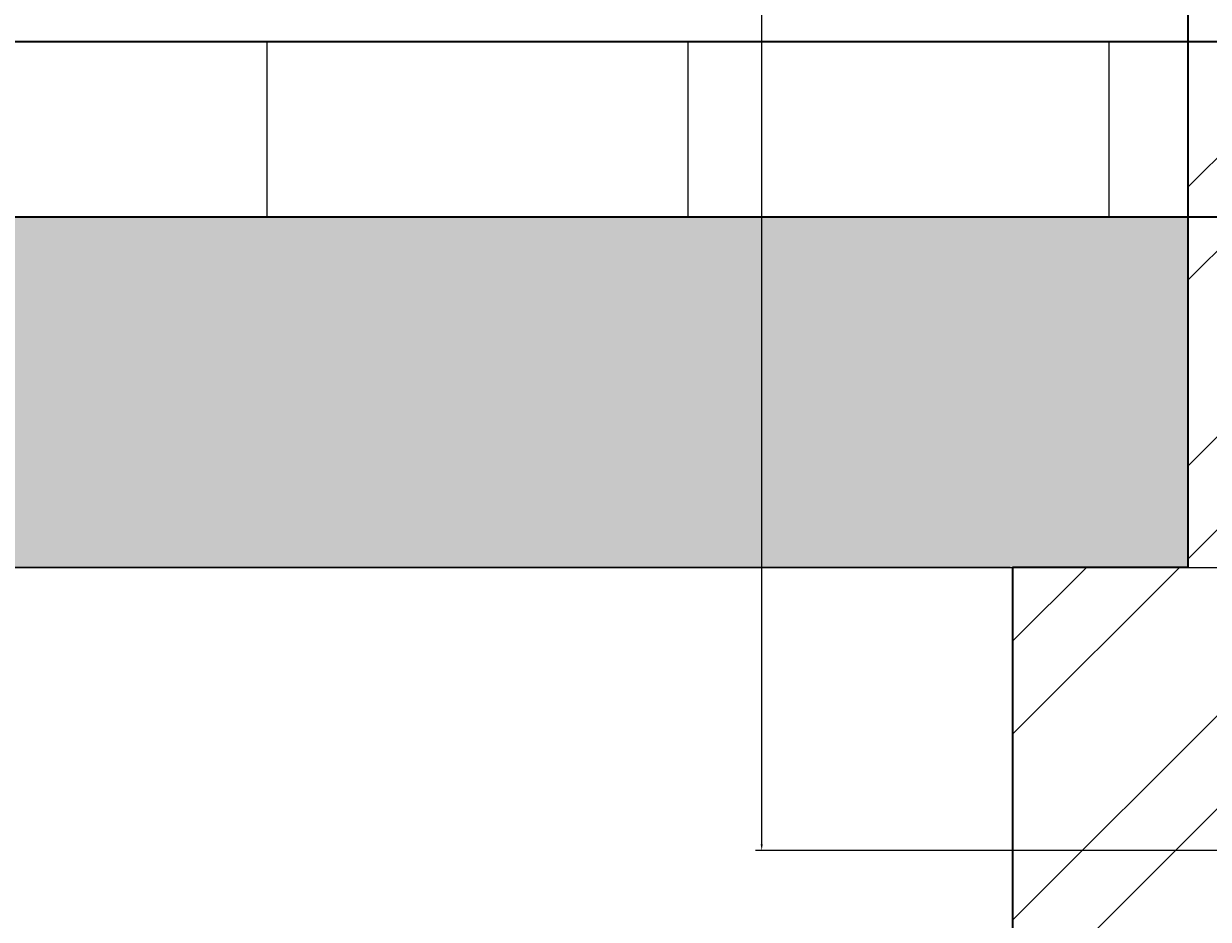
# Model space of a CAD drawing. Units: inches. Extents: x -301 to 715, y -607 to 364.
# Tile 33 of 141: x 101 to 135, y -492 to -466. Entities that reach past the tile are written whole.
import ezdxf

# ---------------------------------------------------------------- set-up
doc = ezdxf.new("R2010")
doc.units = ezdxf.units.IN
doc.header["$MEASUREMENT"] = 0
for name, color, linetype, lineweight in [('A-ANNO-DIMS', 2, 'Continuous', 18), ('A-GRND', 7, 'Continuous', 25), ('A-SECT', 1, 'Continuous', 35), ('A-SECT-PATT', 8, 'Continuous', 13), ('S-FNDN', 2, 'Continuous', 35)]:
    doc.layers.add(name, color=color, linetype=linetype, lineweight=lineweight)
doc.styles.get("Standard").update_dxf_attribs({"font": 'arial.ttf'})
doc.dimstyles.get("Standard").update_dxf_attribs({"dimtxt": 0.18, "dimasz": 0.18, "dimexe": 0.18, "dimexo": 0.0625, "dimgap": 0.09, "dimtad": 0, "dimtih": 1, "dimtoh": 1, "dimdec": 1, "dimzin": 0, "dimdsep": 46, "dimlunit": 4, "dimtxsty": 'Standard', "dimcen": 0.09, "dimclrd": 3, "dimclre": 4, "dimclrt": 6, "dimadec": 0, "dimazin": 0, "dimtfac": 1, "dimtdec": 1, "dimtofl": 0, "dimtmove": 0, "dimatfit": 3, "dimfxl": 1, "dimtfill": 2, "dimtfillclr": 51, "dimtolj": 1, "dimtzin": 0, "dimarcsym": 0})

# ---------------------------------------------------------------- blocks, each defined once
blk = doc.blocks.new('*D176')
at = {"layer": 'A-ANNO-DIMS', "color": 4, "lineweight": -2, "transparency": 16777216}
for p, q in [((148.28, -324.477), (215.605, -324.477)), ((-15.22, -540.477), (215.605, -540.477))]:
    blk.add_line(p, q, dxfattribs=at)
at = {"layer": 'A-ANNO-DIMS', "color": 3, "lineweight": -2, "transparency": 16777216}
for p, q in [((215.425, -324.657), (215.425, -432.296)), ((215.425, -540.297), (215.425, -432.659))]:
    blk.add_line(p, q, dxfattribs=at)
at = {"layer": 'A-ANNO-DIMS', "color": 3, "transparency": 16777216}
for points in [[(215.395, -324.657), (215.455, -324.657), (215.425, -324.477)], [(215.395, -540.297), (215.455, -540.297), (215.425, -540.477)]]:
    blk.add_solid(points, dxfattribs=at)
at = {"layer": 'Defpoints', "color": 0, "transparency": 16777216}
for p in [(148.218, -324.477), (-15.282, -540.477), (215.425, -540.477)]:
    blk.add_point(p, dxfattribs=at)
at = {"layer": 'A-ANNO-DIMS', "color": 6, "transparency": 16777216, "insert": (215.425, -432.477), "char_height": 0.18, "attachment_point": 5, "bg_fill": 1, "box_fill_scale": 1.25, "bg_fill_color": 51, "bg_fill_transparency": 0}
blk.add_mtext('\\A1;18\'-0"', dxfattribs=at)
blk = doc.blocks.new('*D190')
at = {"layer": 'A-ANNO-DIMS', "color": 4, "lineweight": -2, "transparency": 16777216}
for p, q in [((129.193, -481.477), (-266.112, -481.477)), ((124.193, -511.477), (-266.112, -511.477))]:
    blk.add_line(p, q, dxfattribs=at)
at = {"layer": 'A-ANNO-DIMS', "color": 3, "lineweight": -2, "transparency": 16777216}
for p, q in [((-265.932, -481.657), (-265.932, -496.296)), ((-265.932, -511.297), (-265.932, -496.659))]:
    blk.add_line(p, q, dxfattribs=at)
at = {"layer": 'A-ANNO-DIMS', "color": 3, "transparency": 16777216}
for points in [[(-265.962, -481.657), (-265.902, -481.657), (-265.932, -481.477)], [(-265.962, -511.297), (-265.902, -511.297), (-265.932, -511.477)]]:
    blk.add_solid(points, dxfattribs=at)
at = {"layer": 'Defpoints', "color": 0, "transparency": 16777216}
for p in [(129.255, -481.477), (-265.932, -511.477), (124.255, -511.477)]:
    blk.add_point(p, dxfattribs=at)
at = {"layer": 'A-ANNO-DIMS', "color": 6, "transparency": 16777216, "insert": (-265.932, -496.477), "char_height": 0.18, "attachment_point": 5, "bg_fill": 1, "box_fill_scale": 1.25, "bg_fill_color": 51, "bg_fill_transparency": 0}
blk.add_mtext('\\A1;2\'-6"', dxfattribs=at)
blk = doc.blocks.new('*D191')
at = {"layer": 'A-ANNO-DIMS', "color": 4, "lineweight": -2, "transparency": 16777216}
for p, q in [((129.193, -481.477), (-266.112, -481.477)), ((114.193, -540.477), (-266.112, -540.477))]:
    blk.add_line(p, q, dxfattribs=at)
at = {"layer": 'A-ANNO-DIMS', "color": 3, "lineweight": -2, "transparency": 16777216}
for p, q in [((-265.932, -481.657), (-265.932, -510.797)), ((-265.932, -540.297), (-265.932, -511.158))]:
    blk.add_line(p, q, dxfattribs=at)
at = {"layer": 'A-ANNO-DIMS', "color": 3, "transparency": 16777216}
for points in [[(-265.962, -481.657), (-265.902, -481.657), (-265.932, -481.477)], [(-265.962, -540.297), (-265.902, -540.297), (-265.932, -540.477)]]:
    blk.add_solid(points, dxfattribs=at)
at = {"layer": 'Defpoints', "color": 0, "transparency": 16777216}
for p in [(129.255, -481.477), (-265.932, -540.477), (114.255, -540.477)]:
    blk.add_point(p, dxfattribs=at)
at = {"layer": 'A-ANNO-DIMS', "color": 6, "transparency": 16777216, "insert": (-265.932, -510.977), "char_height": 0.18, "attachment_point": 5, "bg_fill": 1, "box_fill_scale": 1.25, "bg_fill_color": 51, "bg_fill_transparency": 0}
blk.add_mtext('\\A1;4\'-11"', dxfattribs=at)
blk = doc.blocks.new('*D200')
at = {"layer": 'A-ANNO-DIMS', "color": 4, "lineweight": -2, "transparency": 16777216}
for p, q in [((412.955, -393.552), (121.926, -393.552)), ((412.955, -489.552), (121.926, -489.552))]:
    blk.add_line(p, q, dxfattribs=at)
at = {"layer": 'A-ANNO-DIMS', "color": 3, "lineweight": -2, "transparency": 16777216}
for p, q in [((122.106, -393.732), (122.106, -441.371)), ((122.106, -489.372), (122.106, -441.734))]:
    blk.add_line(p, q, dxfattribs=at)
at = {"layer": 'A-ANNO-DIMS', "color": 3, "transparency": 16777216}
for points in [[(122.076, -393.732), (122.136, -393.732), (122.106, -393.552)], [(122.076, -489.372), (122.136, -489.372), (122.106, -489.552)]]:
    blk.add_solid(points, dxfattribs=at)
at = {"layer": 'Defpoints', "color": 0, "transparency": 16777216}
for p in [(122.106, -393.552), (413.018, -393.552), (413.018, -489.552)]:
    blk.add_point(p, dxfattribs=at)
at = {"layer": 'A-ANNO-DIMS', "color": 6, "transparency": 16777216, "insert": (122.106, -441.552), "char_height": 0.18, "attachment_point": 5, "bg_fill": 1, "box_fill_scale": 1.25, "bg_fill_color": 51, "bg_fill_transparency": 0}
blk.add_mtext('\\A1;8\'-0"', dxfattribs=at)

msp = doc.modelspace()

# ---------------------------------------------------------------- hatches: boundary and pattern name
at = {"layer": 'A-SECT-PATT'}
h = msp.add_hatch(dxfattribs=at)
h.set_pattern_fill('ANSI32', color=256, scale=15)
h.set_pattern_definition([(45, (10.321, 33.8764), (-3.977476, 3.977476), []), (45, (12.973, 33.8764), (-3.977476, 3.977476), [])])
h.paths.add_polyline_path([(-185.282, -324.477), (-199.282, -324.477), (-199.282, -329.477), (-194.282, -329.477), (-194.282, -353.477), (-185.282, -353.477)])
h.paths.add_polyline_path([(-185.282, -361.477), (-193.904, -361.477), (-193.982, -377.537), (-185.282, -377.537)])
h.paths.add_polyline_path([(143.218, -329.477), (148.218, -329.477), (148.218, -324.477), (134.255, -324.477), (134.255, -353.477), (143.218, -353.477)])
h.paths.add_polyline_path([(143.218, -361.477), (134.255, -361.477), (134.255, -377.477), (143.218, -377.477)])
h.paths.add_polyline_path([(-185.282, -439.477), (-194.282, -439.477), (-194.282, -463.477), (-185.282, -463.477)])
h.paths.add_polyline_path([(-185.282, -471.477), (-194.282, -471.477), (-194.282, -481.477), (-185.282, -481.477)])
h.paths.add_polyline_path([(-185.282, -463.477), (-194.282, -463.477), (-194.282, -466.477), (-185.282, -466.477)])
h.paths.add_polyline_path([(-185.282, -466.477), (-194.282, -466.477), (-194.282, -471.477), (-185.282, -471.477)])
h.paths.add_polyline_path([(-180.282, -481.477), (-185.282, -481.477), (-194.282, -481.477), (-199.282, -481.477), (-199.282, -493.477), (-180.282, -493.477)])
h.paths.add_polyline_path([(-175.282, -493.477), (-180.282, -493.477), (-199.282, -493.477), (-204.282, -493.477), (-204.282, -511.477), (-175.282, -511.477)])
h.paths.add_polyline_path([(-170.282, -511.477), (-175.282, -511.477), (-204.282, -511.477), (-209.282, -511.477), (-209.282, -535.477), (-170.282, -535.477)])
h.paths.add_polyline_path([(-35.282, -463.477), (-41.282, -463.477), (-41.282, -466.477), (-35.282, -466.477)])
h.paths.add_polyline_path([(-35.282, -466.477), (-41.282, -466.477), (-41.282, -471.477), (-35.282, -471.477)])
h.paths.add_polyline_path([(-35.282, -471.477), (-41.282, -471.477), (-41.282, -481.477), (-35.282, -481.477)])
h.paths.add_polyline_path([(-30.282, -481.477), (-46.282, -481.477), (-46.282, -493.477), (-30.282, -493.477)])
h.paths.add_polyline_path([(-25.282, -493.477), (-30.282, -493.477), (-46.282, -493.477), (-51.282, -493.477), (-51.282, -511.477), (-25.282, -511.477)])
h.paths.add_polyline_path([(-20.282, -511.477), (-25.282, -511.477), (-51.282, -511.477), (-56.282, -511.477), (-56.282, -535.477), (-20.282, -535.477)])
h.paths.add_polyline_path([(143.218, -463.477), (134.255, -463.477), (134.255, -466.477), (143.218, -466.477)])
h.paths.add_polyline_path([(143.218, -466.477), (134.255, -466.477), (134.255, -471.477), (143.218, -471.477)])
h.paths.add_polyline_path([(143.218, -471.477), (134.255, -471.477), (134.255, -481.477), (143.218, -481.477)])
h.paths.add_polyline_path([(148.255, -481.477), (143.255, -481.477), (134.255, -481.477), (129.255, -481.477), (129.255, -493.477), (148.255, -493.477)])
h.paths.add_polyline_path([(153.255, -493.477), (148.255, -493.477), (129.255, -493.477), (124.255, -493.477), (124.255, -511.477), (153.255, -511.477)])
h.paths.add_polyline_path([(158.255, -511.477), (153.255, -511.477), (124.255, -511.477), (119.255, -511.477), (119.255, -535.477), (158.255, -535.477)])
h = msp.add_hatch(dxfattribs=at)
h.set_pattern_fill('AR-CONC', color=256, scale=0.5)
h.set_pattern_definition([(50, (10.3213, 33.8764), (3.586301, -0.31376), [0.375, -4.125]), (355, (10.3213, 33.8764), (-0.693757, 3.76096), [0.3, -3.3]), (100.45144, (10.62, 33.8502), (2.892544, 3.4472), [0.3187, -3.50571]), (46.1842, (10.3213, 34.8764), (5.336207, -0.827596), [0.5625, -6.1875]), (96.6356, (10.766, 34.8074), (4.67331, 4.870593), [0.47805, -5.25857]), (351.1842, (10.321, 34.8764), (4.67331, 4.870593), [0.45, -4.95]), (21, (10.8213, 34.6264), (2.984535, -2.013094), [0.375, -4.125]), (326, (10.8213, 34.6264), (1.216577, 3.62575), [0.3, -3.3]), (71.45144, (11.07, 34.4586), (4.201112, 1.612656), [0.3187, -3.50571]), (37.5, (10.3213, 33.8764), (0.0607993, 1.6644693), [0, -3.26, 0, -3.35, 0, -3.3125]), (7.5, (10.3213, 33.8764), (1.3153477, 1.9720586), [0, -1.91, 0, -3.185, 0, -1.2625]), (327.5, (9.2063, 33.8764), (2.6691122, -0.1127744), [0, -1.25, 0, -3.9, 0, -5.175]), (317.5, (8.7063, 33.8764), (2.915931, 0.500525), [0, -1.625, 0, -2.59, 0, -3.675])])
h.paths.add_polyline_path([(-56.282, -535.477), (-61.282, -535.477), (-61.282, -540.477), (-15.282, -540.477), (-15.282, -535.477), (-20.282, -535.477)])
h.paths.add_polyline_path([(119.255, -535.477), (114.255, -535.477), (114.255, -540.477), (163.255, -540.477), (163.255, -535.477), (158.255, -535.477)])
h.paths.add_polyline_path([(-206.282, -471.477), (-209.282, -471.477), (-209.282, -481.477), (-206.282, -481.477), (-194.282, -481.477), (-194.282, -471.477)])
h.paths.add_polyline_path([(-41.282, -481.477), (-41.282, -471.477), (-185.282, -471.477), (-185.282, -481.477), (-180.282, -481.477)])
h.paths.add_polyline_path([(134.255, -481.477), (134.255, -471.477), (-35.282, -471.477), (-35.282, -481.477), (-30.282, -481.477)])
h.paths.add_polyline_path([(155.218, -481.477), (158.218, -481.477), (158.218, -471.477), (153.218, -471.477), (143.218, -471.477), (143.218, -481.477), (148.255, -481.477)])
h.paths.add_polyline_path([(-193.88, -356.477), (-193.904, -361.477), (143.218, -361.477), (143.218, -356.477)])
h = msp.add_hatch(dxfattribs=at)
h.set_pattern_fill('ANSI31', color=256, scale=96, angle=45, style=0)
h.paths.add_polyline_path([(-35.282, -471.477), (134.255, -471.477), (134.255, -466.477), (-35.282, -466.477)])

# ---------------------------------------------------------------- linework, layer by layer
at = {"layer": 'A-GRND'}
msp.add_line((-206.282, -481.477), (155.218, -481.477), dxfattribs=at)
at = {"layer": 'A-SECT'}
for p, q in [((134.255, -361.477), (134.255, -481.477)), ((-204.282, -466.477), (153.218, -466.477)), ((-206.282, -471.477), (155.218, -471.477))]:
    msp.add_line(p, q, dxfattribs=at)
at = {"layer": 'S-FNDN'}
for p, q in [((134.255, -481.477), (129.255, -481.477)), ((129.255, -481.477), (129.255, -493.477))]:
    msp.add_line(p, q, dxfattribs=at)

# ---------------------------------------------------------------- dimensions: what is measured, and where the dimension line sits
at = {"layer": 'A-ANNO-DIMS'}
for base, p1, p2, picture, middle in [((215.425, -540.477), (148.218, -324.477), (-15.282, -540.477), '*D176', (215.425, -432.477)), ((122.106, -393.552), (413.018, -489.552), (413.018, -393.552), '*D200', (122.106, -441.552)), ((-265.932, -540.477), (129.255, -481.477), (114.255, -540.477), '*D191', (-265.932, -510.977)), ((-265.932, -511.477), (129.255, -481.477), (124.255, -511.477), '*D190', (-265.932, -496.477))]:
    dim = msp.add_linear_dim(base=base, p1=p1, p2=p2, angle=90, dimstyle='Standard', override={"dimdec": 1, "dimlfac": 1, "dimrnd": 0, "dimzin": 1, "dimdsep": 46, "dimlunit": 4, "dimfrac": 2}, dxfattribs=at)
    dim.commit()
    dim.dimension.update_dxf_attribs({"geometry": picture, "text_midpoint": middle})

doc.saveas('drawing.dxf')
